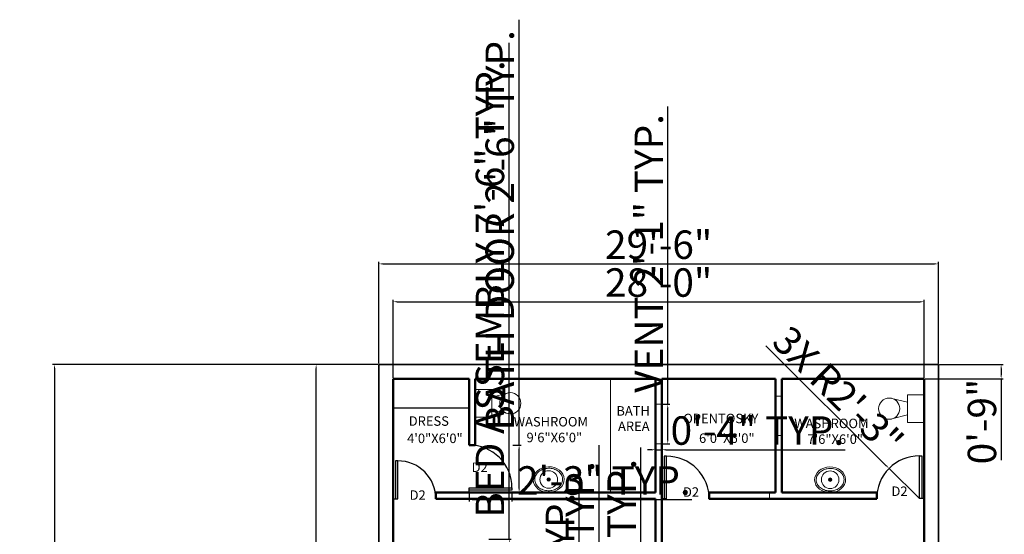
# Model space of a CAD drawing. Units: inches. Extents: x 2040 to 2729, y 1653 to 2621.
# Tile 4 of 4: x 2040 to 2663, y 2295 to 2621. Entities that reach past the tile are written whole.
import ezdxf

# ---------------------------------------------------------------- set-up
doc = ezdxf.new("R2010")
doc.units = ezdxf.units.IN
doc.layers.get('0').update_dxf_attribs({"color": 111})
for name, color, linetype, lineweight in [('A-ANNO-DIMS', 10, 'Continuous', 18), ('A-ANNO-TEXT', 30, 'Continuous', 18), ('A-AREA-IDEN', 6, 'Continuous', 18), ('A-DOOR', 50, 'Continuous', 25), ('A-FLOR-CASE', 30, 'Continuous', 25), ('A-FLOR-FIXT', 4, 'Continuous', 18), ('A-GLAZ', 31, 'Continuous', 18), ('A-WALL', 7, 'Continuous', 50), ('C-PROP', 111, 'Continuous', 35)]:
    doc.layers.add(name, color=color, linetype=linetype, lineweight=lineweight)
doc.styles.get("Standard").update_dxf_attribs({"font": 'arial.ttf'})
doc.dimstyles.new('ISO-25', dxfattribs={"dimtxt": 18, "dimasz": 2.5, "dimexe": 1.25, "dimexo": 0.625, "dimtad": 1, "dimdec": 0, "dimlunit": 3, "dimtxsty": 'Standard', "dimcen": 2.5, "dimadec": 0, "dimazin": 0, "dimtfac": 1, "dimtdec": 0, "dimtmove": 0, "dimatfit": 3, "dimfxl": 1, "dimarcsym": 0})

# ---------------------------------------------------------------- blocks, each defined once
blk = doc.blocks.new('*D5')
at = {"layer": 'A-ANNO-DIMS', "color": 0, "lineweight": -2, "transparency": 16777216}
for p, q in [((2266.85, 2402.66), (2060.98, 2402.66)), ((2062.23, 2400.16), (2062.23, 1697.16)), ((2266.85, 1694.66), (2060.98, 1694.66))]:
    blk.add_line(p, q, dxfattribs=at)
at = {"layer": 'A-ANNO-DIMS', "color": 0, "transparency": 16777216}
for points in [[(2061.81, 2400.16), (2062.64, 2400.16), (2062.23, 2402.66)], [(2061.81, 1697.16), (2062.64, 1697.16), (2062.23, 1694.66)]]:
    blk.add_solid(points, dxfattribs=at)
at = {"layer": 'Defpoints', "color": 0, "transparency": 16777216}
for p in [(2267.47, 2402.66), (2062.23, 1694.66), (2267.47, 1694.66)]:
    blk.add_point(p, dxfattribs=at)
at = {"layer": 'A-ANNO-DIMS', "color": 0, "transparency": 16777216, "insert": (2052.41, 2048.66), "char_height": 18, "attachment_point": 5, "rotation": 90}
blk.add_mtext("59'", dxfattribs=at)
blk = doc.blocks.new('*D6')
at = {"layer": 'A-ANNO-DIMS', "color": 0, "lineweight": -2, "transparency": 16777216}
for p, q in [((2267.47, 2403.29), (2267.47, 2467.6)), ((2621.47, 2403.29), (2621.47, 2467.6)), ((2269.97, 2466.35), (2618.97, 2466.35))]:
    blk.add_line(p, q, dxfattribs=at)
at = {"layer": 'A-ANNO-DIMS', "color": 0, "transparency": 16777216}
for points in [[(2269.97, 2466.76), (2269.97, 2465.93), (2267.47, 2466.35)], [(2618.97, 2466.76), (2618.97, 2465.93), (2621.47, 2466.35)]]:
    blk.add_solid(points, dxfattribs=at)
at = {"layer": 'Defpoints', "color": 0, "transparency": 16777216}
for p in [(2621.47, 2466.35), (2267.47, 2402.66), (2621.47, 2402.66)]:
    blk.add_point(p, dxfattribs=at)
at = {"layer": 'A-ANNO-DIMS', "color": 0, "transparency": 16777216, "insert": (2444.47, 2476.16), "char_height": 18, "attachment_point": 5}
blk.add_mtext('29\'-6"', dxfattribs=at)
blk = doc.blocks.new('WC-FLOOR-MOUNT')
for p, q in [((0, 0), (10.48, 0)), ((0, -17.59), (0, 0)), ((10.48, 0), (10.48, -17.59)), ((10.48, -5), (20.35, -2.32)), ((10.48, -17.59), (0, -17.59)), ((10.48, -12.9), (20.54, -15.32))]:
    blk.add_line(p, q)
blk.add_circle((22.11, -8.8), 6.71)
blk = doc.blocks.new('BASIN-OVAL')
h = blk.add_hatch(color=256)
h.dxf.hatch_style = 1
h.paths.add_polyline_path([(1.14, 0, 1), (-1.14, 0, 1)])
for radius in [5.58, 1.14]:
    blk.add_circle((0, 0), radius)
blk.add_ellipse((0, 0), major_axis=(9.81, 0.23), ratio=0.826688)
blk.add_open_spline([(8.81, 0.21), (8.8, 0.81), (8.69, 1.4), (8.2, 2.81), (7.72, 3.6), (6.41, 5.01), (5.59, 5.62), (3.7, 6.55), (2.64, 6.87), (0.44, 7.17), (-0.7, 7.15), (-2.89, 6.76), (-3.94, 6.39), (-5.79, 5.39), (-6.59, 4.75), (-7.85, 3.29), (-8.3, 2.48), (-8.82, 0.79), (-8.88, -0.08), (-8.62, -1.78), (-8.3, -2.62), (-7.28, -4.16), (-6.59, -4.86), (-4.92, -6.01), (-3.94, -6.46), (-1.83, -7.03), (-0.7, -7.16), (1.53, -7.05), (2.64, -6.83), (4.67, -6.06), (5.59, -5.52), (7.11, -4.23), (7.72, -3.47), (8.55, -1.86), (8.78, -1), (8.82, -0.02), (8.82, 0.09), (8.81, 0.21)], degree=3, knots=[0, 0, 0, 0, 0.259704, 0.259704, 0.633026, 0.633026, 1.006347, 1.006347, 1.379668, 1.379668, 1.752989, 1.752989, 2.12631, 2.12631, 2.499631, 2.499631, 2.872952, 2.872952, 3.246274, 3.246274, 3.619595, 3.619595, 3.992916, 3.992916, 4.366237, 4.366237, 4.739558, 4.739558, 5.112879, 5.112879, 5.486201, 5.486201, 5.859522, 5.859522, 6.232843, 6.232843, 6.283185, 6.283185, 6.283185, 6.283185])
blk = doc.blocks.new('DOOR-27IN')
for p, q in [((0, -3), (0, 0)), ((0, 0), (27, 0)), ((27, -1.5), (0, -1.5)), ((27, 0), (27, -1.5))]:
    blk.add_line(p, q)
blk.add_arc((0, 0), 27, 359.99851, 90.41355)
blk = doc.blocks.new('VENT-WINDOW-25IN')
blk.add_lwpolyline([(0, 0), (4, 0), (4, 25.02), (0, 25.02)], close=True)
blk = doc.blocks.new('*D26')
at = {"layer": 'A-ANNO-DIMS', "color": 0, "lineweight": -2, "transparency": 16777216}
for p, q in [((2394.17, 2208.66), (2394.17, 2322.12)), ((2399.85, 2208.66), (2392.92, 2208.66)), ((2394.17, 2172.16), (2394.17, 2206.16)), ((2399.85, 2169.66), (2392.92, 2169.66))]:
    blk.add_line(p, q, dxfattribs=at)
at = {"layer": 'A-ANNO-DIMS', "color": 0, "transparency": 16777216}
for points in [[(2393.76, 2206.16), (2394.59, 2206.16), (2394.17, 2208.66)], [(2393.76, 2172.16), (2394.59, 2172.16), (2394.17, 2169.66)]]:
    blk.add_solid(points, dxfattribs=at)
at = {"layer": 'Defpoints', "color": 0, "transparency": 16777216}
for p in [(2394.17, 2208.66), (2400.47, 2208.66), (2400.47, 2169.66)]:
    blk.add_point(p, dxfattribs=at)
at = {"layer": 'A-ANNO-DIMS', "color": 0, "transparency": 16777216, "insert": (2384.35, 2266.64), "char_height": 18, "attachment_point": 5, "rotation": 90}
blk.add_mtext('3\'-3" TYP.', dxfattribs=at)
blk = doc.blocks.new('*D27')
at = {"layer": 'A-ANNO-DIMS', "color": 0, "lineweight": -2, "transparency": 16777216}
for p, q in [((2349.97, 2292.24), (2349.97, 2606.15)), ((2337.1, 2292.24), (2351.22, 2292.24)), ((2349.97, 2204.74), (2349.97, 2289.74)), ((2337.1, 2202.24), (2351.22, 2202.24))]:
    blk.add_line(p, q, dxfattribs=at)
at = {"layer": 'A-ANNO-DIMS', "color": 0, "transparency": 16777216}
for points in [[(2349.56, 2289.74), (2350.39, 2289.74), (2349.97, 2292.24)], [(2349.56, 2204.74), (2350.39, 2204.74), (2349.97, 2202.24)]]:
    blk.add_solid(points, dxfattribs=at)
at = {"layer": 'Defpoints', "color": 0, "transparency": 16777216}
for p in [(2336.47, 2292.24), (2349.97, 2292.24), (2336.47, 2202.24)]:
    blk.add_point(p, dxfattribs=at)
at = {"layer": 'A-ANNO-DIMS', "color": 0, "transparency": 16777216, "insert": (2340.04, 2450.44), "char_height": 18, "attachment_point": 5, "rotation": 90}
blk.add_mtext('BED ASSEMBLY 7\'-6" TYP.', dxfattribs=at)
blk = doc.blocks.new('*D31')
at = {"layer": 'A-ANNO-DIMS', "color": 0, "lineweight": -2, "transparency": 16777216}
for p, q in [((2356.18, 2351.71), (2356.18, 2620.86)), ((2352.29, 2351.71), (2357.43, 2351.71)), ((2356.18, 2324.16), (2356.18, 2349.21)), ((2352.29, 2321.66), (2357.43, 2321.66))]:
    blk.add_line(p, q, dxfattribs=at)
at = {"layer": 'A-ANNO-DIMS', "color": 0, "transparency": 16777216}
for points in [[(2355.76, 2349.21), (2356.59, 2349.21), (2356.18, 2351.71)], [(2355.76, 2324.16), (2356.59, 2324.16), (2356.18, 2321.66)]]:
    blk.add_solid(points, dxfattribs=at)
at = {"layer": 'Defpoints', "color": 0, "transparency": 16777216}
for p in [(2351.67, 2351.71), (2356.18, 2351.71), (2351.67, 2321.66)]:
    blk.add_point(p, dxfattribs=at)
at = {"layer": 'A-ANNO-DIMS', "color": 0, "transparency": 16777216, "insert": (2346.24, 2487.54), "char_height": 18, "attachment_point": 5, "rotation": 90}
blk.add_mtext('BATH DOOR 2\'-6" TYP.', dxfattribs=at)
blk = doc.blocks.new('*D32')
at = {"layer": 'A-ANNO-DIMS', "color": 0, "lineweight": -2, "transparency": 16777216}
for p, q in [((2324.47, 2321.04), (2324.47, 2315.9)), ((2351.67, 2321.04), (2351.67, 2315.9)), ((2326.97, 2317.15), (2349.17, 2317.15)), ((2351.67, 2317.15), (2465.44, 2317.15))]:
    blk.add_line(p, q, dxfattribs=at)
at = {"layer": 'A-ANNO-DIMS', "color": 0, "transparency": 16777216}
for points in [[(2326.97, 2317.57), (2326.97, 2316.74), (2324.47, 2317.15)], [(2349.17, 2317.57), (2349.17, 2316.74), (2351.67, 2317.15)]]:
    blk.add_solid(points, dxfattribs=at)
at = {"layer": 'Defpoints', "color": 0, "transparency": 16777216}
for p in [(2324.47, 2321.66), (2351.67, 2321.66), (2351.67, 2317.15)]:
    blk.add_point(p, dxfattribs=at)
at = {"layer": 'A-ANNO-DIMS', "color": 0, "transparency": 16777216, "insert": (2409.81, 2326.97), "char_height": 18, "attachment_point": 5}
blk.add_mtext('2\'-3" TYP.', dxfattribs=at)
blk = doc.blocks.new('*D33')
at = {"layer": 'A-ANNO-DIMS', "color": 0, "lineweight": -2, "transparency": 16777216}
for p, q in [((2406.86, 2019.66), (2406.86, 2351.67)), ((2401.19, 2019.66), (2408.11, 2019.66)), ((2406.86, 1980.16), (2406.86, 2017.16)), ((2401.19, 1977.66), (2408.11, 1977.66))]:
    blk.add_line(p, q, dxfattribs=at)
at = {"layer": 'A-ANNO-DIMS', "color": 0, "transparency": 16777216}
for points in [[(2406.45, 2017.16), (2407.28, 2017.16), (2406.86, 2019.66)], [(2406.45, 1980.16), (2407.28, 1980.16), (2406.86, 1977.66)]]:
    blk.add_solid(points, dxfattribs=at)
at = {"layer": 'Defpoints', "color": 0, "transparency": 16777216}
for p in [(2400.56, 2019.66), (2406.86, 2019.66), (2400.56, 1977.66)]:
    blk.add_point(p, dxfattribs=at)
at = {"layer": 'A-ANNO-DIMS', "color": 0, "transparency": 16777216, "insert": (2396.92, 2186.92), "char_height": 18, "attachment_point": 5, "rotation": 90}
blk.add_mtext('BEDROOM DOOR 3\'-6" TYP.', dxfattribs=at)
blk = doc.blocks.new('*D37')
at = {"layer": 'A-ANNO-DIMS', "color": 0, "lineweight": -2, "transparency": 16777216}
for p, q in [((2450.23, 2377.49), (2450.23, 2565.95)), ((2447.1, 2377.49), (2451.48, 2377.49)), ((2450.23, 2354.98), (2450.23, 2374.99)), ((2447.1, 2352.48), (2451.48, 2352.48))]:
    blk.add_line(p, q, dxfattribs=at)
at = {"layer": 'A-ANNO-DIMS', "color": 0, "transparency": 16777216}
for points in [[(2449.81, 2374.99), (2450.64, 2374.99), (2450.23, 2377.49)], [(2449.81, 2354.98), (2450.64, 2354.98), (2450.23, 2352.48)]]:
    blk.add_solid(points, dxfattribs=at)
at = {"layer": 'Defpoints', "color": 0, "transparency": 16777216}
for p in [(2446.47, 2377.49), (2450.23, 2377.49), (2446.47, 2352.48)]:
    blk.add_point(p, dxfattribs=at)
at = {"layer": 'A-ANNO-DIMS', "color": 0, "transparency": 16777216, "insert": (2440.56, 2472.97), "char_height": 18, "attachment_point": 5, "rotation": 90}
blk.add_mtext('VENT 2\'-1" TYP.', dxfattribs=at)
blk = doc.blocks.new('*D38')
at = {"layer": 'A-ANNO-DIMS', "color": 0, "lineweight": -2, "transparency": 16777216}
for p, q in [((2442.47, 2351.85), (2442.47, 2347.47)), ((2446.47, 2351.85), (2446.47, 2347.47)), ((2439.97, 2348.72), (2437.47, 2348.72)), ((2442.47, 2348.72), (2446.47, 2348.72)), ((2448.97, 2348.72), (2562.44, 2348.72))]:
    blk.add_line(p, q, dxfattribs=at)
at = {"layer": 'A-ANNO-DIMS', "color": 0, "transparency": 16777216}
for points in [[(2439.97, 2349.14), (2439.97, 2348.31), (2442.47, 2348.72)], [(2448.97, 2349.14), (2448.97, 2348.31), (2446.47, 2348.72)]]:
    blk.add_solid(points, dxfattribs=at)
at = {"layer": 'Defpoints', "color": 0, "transparency": 16777216}
for p in [(2442.47, 2352.48), (2446.47, 2352.48), (2446.47, 2348.72)]:
    blk.add_point(p, dxfattribs=at)
at = {"layer": 'A-ANNO-DIMS', "color": 0, "transparency": 16777216, "insert": (2506.96, 2358.54), "char_height": 18, "attachment_point": 5}
blk.add_mtext('0\'-4" TYP.', dxfattribs=at)
blk = doc.blocks.new('*D39')
at = {"layer": 'A-ANNO-DIMS', "color": 0, "lineweight": -2, "transparency": 16777216}
for p, q in [((2433.3, 2078.37), (2433.3, 2350.18)), ((2434.21, 2078.37), (2432.05, 2078.37)), ((2433.3, 2070.64), (2433.3, 2075.87)), ((2434.21, 2068.14), (2432.05, 2068.14))]:
    blk.add_line(p, q, dxfattribs=at)
at = {"layer": 'A-ANNO-DIMS', "color": 0, "transparency": 16777216}
for points in [[(2432.88, 2075.87), (2433.72, 2075.87), (2433.3, 2078.37)], [(2432.88, 2070.64), (2433.72, 2070.64), (2433.3, 2068.14)]]:
    blk.add_solid(points, dxfattribs=at)
at = {"layer": 'Defpoints', "color": 0, "transparency": 16777216}
for p in [(2433.3, 2078.37), (2434.84, 2078.37), (2434.84, 2068.14)]:
    blk.add_point(p, dxfattribs=at)
at = {"layer": 'A-ANNO-DIMS', "color": 0, "transparency": 16777216, "insert": (2423.37, 2215.52), "char_height": 18, "attachment_point": 5, "rotation": 90}
blk.add_mtext('END CHAIR 0\'-10" TYP.', dxfattribs=at)
blk = doc.blocks.new('*D41')
at = {"layer": 'A-ANNO-DIMS', "color": 0, "lineweight": -2, "transparency": 16777216}
for p, q in [((2266.85, 2402.66), (2226.49, 2402.66)), ((2227.74, 1775.16), (2227.74, 2400.16)), ((2275.85, 1772.66), (2226.49, 1772.66))]:
    blk.add_line(p, q, dxfattribs=at)
at = {"layer": 'A-ANNO-DIMS', "color": 0, "transparency": 16777216}
for points in [[(2227.33, 2400.16), (2228.16, 2400.16), (2227.74, 2402.66)], [(2227.33, 1775.16), (2228.16, 1775.16), (2227.74, 1772.66)]]:
    blk.add_solid(points, dxfattribs=at)
at = {"layer": 'Defpoints', "color": 0, "transparency": 16777216}
for p in [(2227.74, 2402.66), (2267.47, 2402.66), (2276.47, 1772.66)]:
    blk.add_point(p, dxfattribs=at)
at = {"layer": 'A-ANNO-DIMS', "color": 0, "transparency": 16777216, "insert": (2217.93, 2087.66), "char_height": 18, "attachment_point": 5, "rotation": 90}
blk.add_mtext('52\'-6"', dxfattribs=at)
blk = doc.blocks.new('*D42')
at = {"layer": 'A-ANNO-DIMS', "color": 0, "lineweight": -2, "transparency": 16777216}
for p, q in [((2276.47, 2394.29), (2276.47, 2443.64)), ((2278.97, 2442.39), (2609.97, 2442.39)), ((2612.47, 2394.29), (2612.47, 2443.64))]:
    blk.add_line(p, q, dxfattribs=at)
at = {"layer": 'A-ANNO-DIMS', "color": 0, "transparency": 16777216}
for points in [[(2278.97, 2442.81), (2278.97, 2441.97), (2276.47, 2442.39)], [(2609.97, 2442.81), (2609.97, 2441.97), (2612.47, 2442.39)]]:
    blk.add_solid(points, dxfattribs=at)
at = {"layer": 'Defpoints', "color": 0, "transparency": 16777216}
for p in [(2612.47, 2442.39), (2276.47, 2393.66), (2612.47, 2393.66)]:
    blk.add_point(p, dxfattribs=at)
at = {"layer": 'A-ANNO-DIMS', "color": 0, "transparency": 16777216, "insert": (2444.47, 2452.21), "char_height": 18, "attachment_point": 5}
blk.add_mtext('28\'-0"', dxfattribs=at)
blk = doc.blocks.new('*D43')
at = {"layer": 'A-ANNO-DIMS', "color": 0, "lineweight": -2, "transparency": 16777216}
for p, q in [((2622.1, 2402.66), (2662.45, 2402.66)), ((2661.2, 2400.16), (2661.2, 2396.16)), ((2613.1, 2393.66), (2662.45, 2393.66)), ((2661.2, 2393.66), (2661.2, 2342.06))]:
    blk.add_line(p, q, dxfattribs=at)
at = {"layer": 'A-ANNO-DIMS', "color": 0, "transparency": 16777216}
for points in [[(2660.79, 2400.16), (2661.62, 2400.16), (2661.2, 2402.66)], [(2660.79, 2396.16), (2661.62, 2396.16), (2661.2, 2393.66)]]:
    blk.add_solid(points, dxfattribs=at)
at = {"layer": 'Defpoints', "color": 0, "transparency": 16777216}
for p in [(2621.47, 2402.66), (2612.47, 2393.66), (2661.2, 2393.66)]:
    blk.add_point(p, dxfattribs=at)
at = {"layer": 'A-ANNO-DIMS', "color": 0, "transparency": 16777216, "insert": (2651.39, 2366.61), "char_height": 18, "attachment_point": 5, "rotation": 90}
blk.add_mtext('0\'-9"', dxfattribs=at)
blk = doc.blocks.new('*D51')
at = {"layer": 'A-ANNO-DIMS', "color": 0, "lineweight": -2, "transparency": 16777216}
for p, q in [((2512.26, 2414.4), (2588.54, 2338.66)), ((2609.47, 2317.88), (2590.31, 2336.9))]:
    blk.add_line(p, q, dxfattribs=at)
at = {"layer": 'A-ANNO-DIMS', "color": 0, "transparency": 16777216}
blk.add_solid([(2588.83, 2338.96), (2588.25, 2338.37), (2590.31, 2336.9)], dxfattribs=at)
at = {"layer": 'Defpoints', "color": 0, "transparency": 16777216}
for p in [(2590.31, 2336.9), (2609.47, 2317.88)]:
    blk.add_point(p, dxfattribs=at)
at = {"layer": 'A-ANNO-DIMS', "color": 0, "transparency": 16777216, "insert": (2556.43, 2384.38), "char_height": 18, "attachment_point": 5, "rotation": 315.20528}
blk.add_mtext('3X R2\'-3"', dxfattribs=at)

msp = doc.modelspace()

# ---------------------------------------------------------------- linework, layer by layer
at = {"layer": 'A-DOOR'}
for p, q in [((2447.97, 2344.65), (2447.97, 2317.65)), ((2449.47, 2344.65), (2447.97, 2344.65)), ((2447.97, 2344.65), (2447.97, 2317.65)), ((2449.47, 2317.65), (2449.47, 2344.65)), ((2279.47, 2341.71), (2277.97, 2341.71)), ((2277.97, 2341.71), (2277.97, 2317.71)), ((2279.47, 2317.71), (2279.47, 2341.71)), ((2276.47, 2317.71), (2279.47, 2317.71)), ((2449.47, 2317.65), (2446.47, 2317.65)), ((2446.47, 2317.65), (2449.47, 2317.65))]:
    msp.add_line(p, q, dxfattribs=at)
for centre, radius, start, end in [((2449.47, 2317.65), 27, 359.58645, 90.00149), ((2279.47, 2317.71), 24, 359.8734, 90.00014)]:
    msp.add_arc(centre, radius, start, end, dxfattribs=at)
at = {"layer": 'A-FLOR-CASE'}
msp.add_line((2276.47, 2375.32), (2324.47, 2375.32), dxfattribs=at)
at = {"layer": 'A-FLOR-FIXT'}
for p, q in [((2414.07, 2321.66), (2414.07, 2393.66)), ((2595, 2380.51), (2595, 2379.58)), ((2595, 2369.87), (2595, 2369.02))]:
    msp.add_line(p, q, dxfattribs=at)
at = {"layer": 'A-GLAZ'}
msp.add_lwpolyline([(2476.47, 2317.66), (2514.6, 2317.66), (2514.6, 2321.66), (2476.47, 2321.66)], close=True, dxfattribs=at)
at = {"layer": 'A-WALL'}
for p, q in [((2276.47, 2393.66), (2324.47, 2393.66)), ((2276.47, 1977.66), (2276.47, 2393.66)), ((2324.47, 2351.66), (2324.47, 2393.66)), ((2328.47, 2351.66), (2328.47, 2393.66)), ((2328.47, 2393.66), (2442.47, 2393.66)), ((2442.47, 2321.66), (2442.47, 2393.66)), ((2446.47, 2169.66), (2446.47, 2393.66)), ((2446.47, 2393.66), (2518.47, 2393.66)), ((2518.47, 2321.66), (2518.47, 2393.66)), ((2522.47, 2321.66), (2522.47, 2393.66)), ((2522.47, 2393.66), (2612.47, 2393.66)), ((2612.47, 2393.66), (2612.47, 2173.66)), ((2324.47, 2351.66), (2328.47, 2351.66)), ((2303.47, 2321.66), (2442.47, 2321.66)), ((2303.47, 2317.66), (2303.47, 2321.66)), ((2476.47, 2321.66), (2518.47, 2321.66)), ((2476.47, 2317.66), (2476.47, 2321.66)), ((2522.47, 2321.66), (2582.47, 2321.66)), ((2582.47, 2321.66), (2582.47, 2317.66)), ((2303.47, 2317.66), (2442.47, 2317.66)), ((2442.47, 2169.66), (2442.47, 2317.66)), ((2476.47, 2317.66), (2582.47, 2317.66))]:
    msp.add_line(p, q, dxfattribs=at)
at = {"layer": 'C-PROP'}
msp.add_lwpolyline([(2267.47, 2402.66), (2621.47, 2402.66), (2621.47, 1694.66), (2267.47, 1694.66)], close=True, dxfattribs=at)

# ---------------------------------------------------------------- block references
at = {"layer": 'A-DOOR'}
msp.add_blockref('DOOR-27IN', (2324.67, 2324.66), dxfattribs=at)
at = {"layer": 'A-DOOR', "rotation": 89.99999999999751}
msp.add_blockref('DOOR-27IN', (2609.47, 2317.88), dxfattribs=at)
at = {"layer": 'A-FLOR-FIXT'}
for name, p in [('WC-FLOOR-MOUNT', (2328.47, 2386.96)), ('BASIN-OVAL', (2374.9, 2329.9)), ('BASIN-OVAL', (2553, 2329.78))]:
    msp.add_blockref(name, p, dxfattribs=at)
at = {"layer": 'A-FLOR-FIXT', "rotation": 180}
msp.add_blockref('WC-FLOOR-MOUNT', (2612.47, 2365.93), dxfattribs=at)
at = {"layer": 'A-GLAZ'}
for p in [(2518.47, 2357.66), (2442.47, 2352.48)]:
    msp.add_blockref('VENT-WINDOW-25IN', p, dxfattribs=at)

# ---------------------------------------------------------------- texts
at = {"layer": 'A-ANNO-TEXT'}
for p in [(2326.15, 2334.65), (2459.87, 2318.98), (2591.81, 2319.48), (2286.89, 2317.05)]:
    msp.add_attdef('D2', p, '', height=6, dxfattribs=at)
at = {"layer": 'A-AREA-IDEN'}
for tag, p in [('BATH', (2417.71, 2370.33)), ('DRESS', (2286.34, 2363.9)), ('WASHROOM', (2352.77, 2363.46)), ('OPENTOSKY', (2460.04, 2365.51)), ('WASHROOM', (2530.3, 2362.39)), ('AREA', (2418.75, 2360.6)), ('4\'0"X6\'0"', (2285.3, 2352.95)), ('9\'6"X6\'0"', (2360.87, 2353.49)), ('6\'0"X6\'0"', (2470.02, 2353.05)), ('7\'6"X6\'0"', (2538.62, 2352.42))]:
    msp.add_attdef(tag, p, '', height=6, dxfattribs=at)

# ---------------------------------------------------------------- dimensions: what is measured, and where the dimension line sits
at = {"layer": 'A-ANNO-DIMS'}
for base, p1, p2, text, picture, middle in [((2356.1765, 2351.7132), (2351.6687, 2321.6612), (2351.6687, 2351.7132), 'BATH DOOR <> TYP.', '*D31', (2346.2384, 2487.536)), ((2349.97, 2292.24), (2336.47, 2202.24), (2336.47, 2292.24), 'BED ASSEMBLY <> TYP.', '*D27', (2340.04, 2450.44)), ((2450.23, 2377.49), (2446.47, 2352.48), (2446.47, 2377.49), 'VENT <> TYP.', '*D37', (2440.56, 2472.97)), ((2406.86, 2019.66), (2400.56, 1977.66), (2400.56, 2019.66), 'BEDROOM DOOR <> TYP.', '*D33', (2396.92, 2186.92)), ((2433.3, 2078.37), (2434.84, 2068.14), (2434.84, 2078.37), 'END CHAIR <> TYP.', '*D39', (2423.37, 2215.52)), ((2394.17, 2208.66), (2400.47, 2169.66), (2400.47, 2208.66), '<> TYP.', '*D26', (2384.35, 2266.64))]:
    dim = msp.add_linear_dim(base=base, p1=p1, p2=p2, angle=90, text=text, dimstyle='ISO-25', override={"dimdec": 1, "dimlfac": 1, "dimrnd": 0, "dimzin": 1, "dimdsep": 46, "dimlunit": 4, "dimfrac": 2}, dxfattribs=at)
    dim.commit()
    dim.dimension.update_dxf_attribs({"geometry": picture, "text_midpoint": middle})
for base, p1, p2, override, picture, middle in [((2621.47, 2466.35), (2267.47, 2402.66), (2621.47, 2402.66), {"dimclrd": 0, "dimclre": 0, "dimclrt": 0}, '*D6', (2444.47, 2476.16)), ((2612.47, 2442.39), (2276.47, 2393.66), (2612.47, 2393.66), {"dimdec": 1, "dimlfac": 1, "dimrnd": 0, "dimzin": 1, "dimdsep": 46, "dimlunit": 4, "dimfrac": 2}, '*D42', (2444.47, 2452.21))]:
    dim = msp.add_linear_dim(base=base, p1=p1, p2=p2, dimstyle='ISO-25', override=override, dxfattribs=at)
    dim.commit()
    dim.dimension.update_dxf_attribs({"geometry": picture, "text_midpoint": middle})
dim = msp.add_radius_dim(center=(2609.47, 2317.88), mpoint=(2590.31, 2336.9), text='3X <>', dimstyle='ISO-25', override={"dimdec": 1, "dimlfac": 1, "dimrnd": 0, "dimzin": 1, "dimdsep": 46, "dimlunit": 4, "dimfrac": 2}, dxfattribs=at)
dim.commit()
dim.dimension.update_dxf_attribs({"geometry": '*D51', "text_midpoint": (2556.43, 2384.38)})
for base, p1, p2, override, picture, middle in [((2062.23, 1694.66), (2267.47, 2402.66), (2267.47, 1694.66), {"dimclrd": 0, "dimclre": 0, "dimclrt": 0}, '*D5', (2052.41, 2048.66)), ((2227.74, 2402.66), (2276.47, 1772.66), (2267.47, 2402.66), {"dimdec": 1, "dimlfac": 1, "dimrnd": 0, "dimzin": 1, "dimdsep": 46, "dimlunit": 4, "dimfrac": 2}, '*D41', (2217.93, 2087.66)), ((2661.2, 2393.66), (2621.47, 2402.66), (2612.47, 2393.66), {"dimdec": 1, "dimlfac": 1, "dimrnd": 0, "dimzin": 1, "dimdsep": 46, "dimlunit": 4, "dimfrac": 2}, '*D43', (2651.39, 2366.61))]:
    dim = msp.add_linear_dim(base=base, p1=p1, p2=p2, angle=90, dimstyle='ISO-25', override=override, dxfattribs=at)
    dim.commit()
    dim.dimension.update_dxf_attribs({"geometry": picture, "text_midpoint": middle})
for base, p1, p2, picture, middle in [((2446.47, 2348.72), (2442.47, 2352.48), (2446.47, 2352.48), '*D38', (2506.96, 2358.54)), ((2351.67, 2317.15), (2324.47, 2321.66), (2351.67, 2321.66), '*D32', (2409.81, 2326.97))]:
    dim = msp.add_linear_dim(base=base, p1=p1, p2=p2, text='<> TYP.', dimstyle='ISO-25', override={"dimdec": 1, "dimlfac": 1, "dimrnd": 0, "dimzin": 1, "dimdsep": 46, "dimlunit": 4, "dimfrac": 2}, dxfattribs=at)
    dim.commit()
    dim.dimension.update_dxf_attribs({"geometry": picture, "text_midpoint": middle})

doc.saveas('drawing.dxf')
